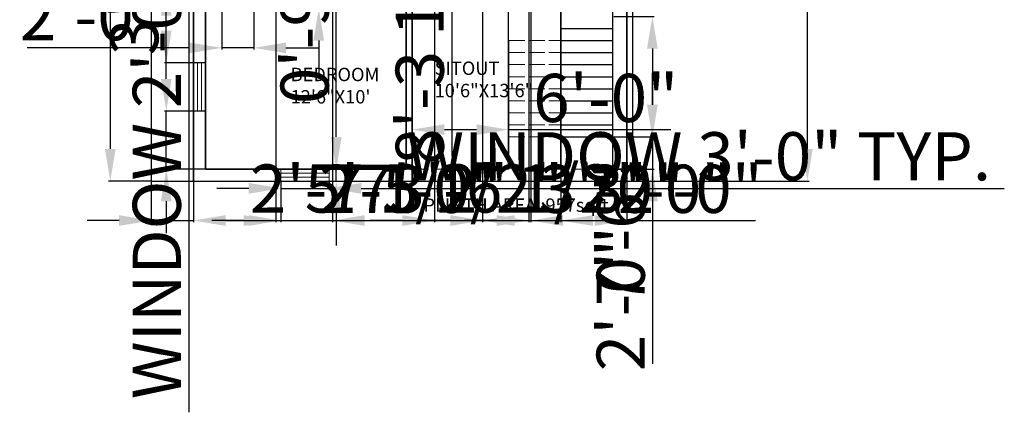
# Model space of a CAD drawing. Units: inches. Extents: x 1041 to 1781, y -140 to 732.
# Tile 1 of 6: x 1045 to 1781, y -140 to 153. Entities that reach past the tile are written whole.
import ezdxf

# ---------------------------------------------------------------- set-up
doc = ezdxf.new("R2010")
doc.units = ezdxf.units.IN
doc.linetypes.add('ACAD_ISO02W100', pattern=[15, 12, -3])
for name, color, linetype, lineweight in [('A-ANNO-TEXT', 7, 'Continuous', 18), ('A-AREA-IDEN', 7, 'Continuous', 20), ('A-FLOR', 7, 'Continuous', 25), ('A-FLOR-HIDN', 7, 'ACAD_ISO02W100', 18), ('A-FLOR-STRS', 7, 'Continuous', 25), ('A-FLOR-STRS-OVHD', 7, 'ACAD_ISO02W100', 18), ('A-GLAZ', 4, 'Continuous', 18), ('A-WALL', 7, 'Continuous', 35), ('C-PROP', 3, 'Continuous', 25), ('dimension', 130, 'Continuous', 18)]:
    doc.layers.add(name, color=color, linetype=linetype, lineweight=lineweight)
doc.styles.get("Standard").update_dxf_attribs({"font": 'arial.ttf'})
doc.dimstyles.new('ISO-25', dxfattribs={"dimtxt": 36, "dimasz": 24, "dimexe": 1.25, "dimexo": 0.625, "dimtad": 1, "dimlunit": 4, "dimtxsty": 'Standard', "dimcen": 2.5, "dimadec": 0, "dimazin": 0, "dimtfac": 1, "dimtmove": 0, "dimatfit": 3, "dimfxl": 1, "dimarcsym": 0})

# ---------------------------------------------------------------- blocks, each defined once
blk = doc.blocks.new('*D2')
at = {"layer": 'Defpoints', "color": 0, "transparency": 16777216}
for p in [(1143.25, 512.23), (1112.63, 32.23), (1143.25, 32.23)]:
    blk.add_point(p, dxfattribs=at)
at = {"layer": 'dimension', "color": 0, "lineweight": -2, "transparency": 16777216}
for p, q in [((1142.62, 512.23), (1111.38, 512.23)), ((1112.63, 488.23), (1112.63, 56.23)), ((1142.62, 32.23), (1111.38, 32.23))]:
    blk.add_line(p, q, dxfattribs=at)
at = {"layer": 'dimension', "color": 0, "transparency": 16777216}
for points in [[(1108.63, 488.23), (1116.63, 488.23), (1112.63, 512.23)], [(1108.63, 56.23), (1116.63, 56.23), (1112.63, 32.23)]]:
    blk.add_solid(points, dxfattribs=at)
at = {"layer": 'dimension', "color": 0, "transparency": 16777216, "insert": (1093.62, 272.23), "char_height": 36, "attachment_point": 5, "rotation": 90}
blk.add_mtext("40'", dxfattribs=at)
blk = doc.blocks.new('WIN-36IN')
for p, q in [((0, 9), (0, 0)), ((36, 9), (0, 9)), ((36, 0), (36, 9)), ((36, 6), (0, 6)), ((0, 3), (36, 3)), ((0, 0), (36, 0)), ((0, 0), (36, 0))]:
    blk.add_line(p, q)
blk = doc.blocks.new('*D9')
at = {"layer": 'Defpoints', "color": 0, "transparency": 16777216}
for p in [(1174.94, 388.32), (1171.34, 364.32), (1174.94, 364.32)]:
    blk.add_point(p, dxfattribs=at)
at = {"layer": 'dimension', "color": 0, "lineweight": -2, "transparency": 16777216}
for p, q in [((1171.34, 412.32), (1171.34, 436.32)), ((1174.31, 388.32), (1170.09, 388.32)), ((1171.34, 388.32), (1171.34, 364.32)), ((1174.31, 364.32), (1170.09, 364.32)), ((1171.34, 340.32), (1171.34, -140.48))]:
    blk.add_line(p, q, dxfattribs=at)
at = {"layer": 'dimension', "color": 0, "transparency": 16777216}
for points in [[(1167.34, 412.32), (1175.34, 412.32), (1171.34, 388.32)], [(1167.34, 340.32), (1175.34, 340.32), (1171.34, 364.32)]]:
    blk.add_solid(points, dxfattribs=at)
at = {"layer": 'dimension', "color": 0, "transparency": 16777216, "insert": (1152.09, 87.92), "char_height": 36, "attachment_point": 5, "rotation": 90}
blk.add_mtext('WINDOW 2\'-0" TYP.', dxfattribs=at)
blk = doc.blocks.new('*D11')
at = {"layer": 'Defpoints', "color": 0, "transparency": 16777216}
for p in [(1240.2, 32.23), (1276.2, 32.23), (1276.2, 26.83)]:
    blk.add_point(p, dxfattribs=at)
at = {"layer": 'dimension', "color": 0, "lineweight": -2, "transparency": 16777216}
for p, q in [((1240.2, 31.61), (1240.2, 25.58)), ((1276.2, 31.61), (1276.2, 25.58)), ((1216.2, 26.83), (1192.2, 26.83)), ((1240.2, 26.83), (1276.2, 26.83)), ((1300.2, 26.83), (1781, 26.83))]:
    blk.add_line(p, q, dxfattribs=at)
at = {"layer": 'dimension', "color": 0, "transparency": 16777216}
for points in [[(1216.2, 30.83), (1216.2, 22.83), (1240.2, 26.83)], [(1300.2, 30.83), (1300.2, 22.83), (1276.2, 26.83)]]:
    blk.add_solid(points, dxfattribs=at)
at = {"layer": 'dimension', "color": 0, "transparency": 16777216, "insert": (1552.6, 46.1), "char_height": 36, "attachment_point": 5}
blk.add_mtext('WINDOW 3\'-0" TYP.', dxfattribs=at)
blk = doc.blocks.new('*D12')
at = {"layer": 'Defpoints', "color": 0, "transparency": 16777216}
for p in [(1276.2, 41.23), (1281.6, 41.23), (1276.2, 32.23)]:
    blk.add_point(p, dxfattribs=at)
at = {"layer": 'dimension', "color": 0, "lineweight": -2, "transparency": 16777216}
for p, q in [((1281.6, 65.23), (1281.6, 309.92)), ((1276.83, 41.23), (1282.85, 41.23)), ((1281.6, 32.23), (1281.6, 41.23)), ((1276.83, 32.23), (1282.85, 32.23)), ((1281.6, 8.23), (1281.6, -15.77))]:
    blk.add_line(p, q, dxfattribs=at)
at = {"layer": 'dimension', "color": 0, "transparency": 16777216}
for points in [[(1277.6, 65.23), (1285.6, 65.23), (1281.6, 41.23)], [(1277.6, 8.23), (1285.6, 8.23), (1281.6, 32.23)]]:
    blk.add_solid(points, dxfattribs=at)
at = {"layer": 'dimension', "color": 0, "transparency": 16777216, "insert": (1262.59, 199.58), "char_height": 36, "attachment_point": 5, "rotation": 90}
blk.add_mtext('0\'-9" TYP.', dxfattribs=at)
blk = doc.blocks.new('*D15')
at = {"layer": 'Defpoints', "color": 0, "transparency": 16777216}
for p in [(1174.94, 32.23), (1498.75, 32.23), (1498.75, 2.78)]:
    blk.add_point(p, dxfattribs=at)
at = {"layer": 'dimension', "color": 0, "lineweight": -2, "transparency": 16777216}
for p, q in [((1174.94, 31.61), (1174.94, 1.53)), ((1498.75, 31.61), (1498.75, 1.53)), ((1198.94, 2.78), (1474.75, 2.78))]:
    blk.add_line(p, q, dxfattribs=at)
at = {"layer": 'dimension', "color": 0, "transparency": 16777216}
for points in [[(1198.94, 6.78), (1198.94, -1.22), (1174.94, 2.78)], [(1474.75, 6.78), (1474.75, -1.22), (1498.75, 2.78)]]:
    blk.add_solid(points, dxfattribs=at)
at = {"layer": 'dimension', "color": 0, "transparency": 16777216, "insert": (1336.84, 21.79), "char_height": 36, "attachment_point": 5}
blk.add_mtext('27\'-0"', dxfattribs=at)
blk = doc.blocks.new('*D16')
at = {"layer": 'Defpoints', "color": 0, "transparency": 16777216}
for p in [(1498.75, 503.23), (1633.79, 503.23), (1498.75, 32.23)]:
    blk.add_point(p, dxfattribs=at)
at = {"layer": 'dimension', "color": 0, "lineweight": -2, "transparency": 16777216}
for p, q in [((1499.37, 503.23), (1635.04, 503.23)), ((1633.79, 56.23), (1633.79, 479.23)), ((1499.37, 32.23), (1635.04, 32.23))]:
    blk.add_line(p, q, dxfattribs=at)
at = {"layer": 'dimension', "color": 0, "transparency": 16777216}
for points in [[(1629.79, 479.23), (1637.79, 479.23), (1633.79, 503.23)], [(1629.79, 56.23), (1637.79, 56.23), (1633.79, 32.23)]]:
    blk.add_solid(points, dxfattribs=at)
at = {"layer": 'dimension', "color": 0, "transparency": 16777216, "insert": (1614.78, 267.73), "char_height": 36, "attachment_point": 5, "rotation": 90}
blk.add_mtext('39\'-3"', dxfattribs=at)
blk = doc.blocks.new('*D17')
at = {"layer": 'Defpoints', "color": 0, "transparency": 16777216}
for p in [(1143.25, 32.23), (1174.94, 32.23), (1174.94, 2.78)]:
    blk.add_point(p, dxfattribs=at)
at = {"layer": 'dimension', "color": 0, "lineweight": -2, "transparency": 16777216}
for p, q in [((1143.25, 31.61), (1143.25, 1.53)), ((1174.94, 31.61), (1174.94, 1.53)), ((1119.25, 2.78), (1095.25, 2.78)), ((1143.25, 2.78), (1174.94, 2.78)), ((1198.94, 2.78), (1404.38, 2.78))]:
    blk.add_line(p, q, dxfattribs=at)
at = {"layer": 'dimension', "color": 0, "transparency": 16777216}
for points in [[(1119.25, 6.78), (1119.25, -1.22), (1143.25, 2.78)], [(1198.94, 6.78), (1198.94, -1.22), (1174.94, 2.78)]]:
    blk.add_solid(points, dxfattribs=at)
at = {"layer": 'dimension', "color": 0, "transparency": 16777216, "insert": (1313.66, 22.02), "char_height": 36, "attachment_point": 5}
blk.add_mtext('2\'-7 1/2"', dxfattribs=at)
blk = doc.blocks.new('*D19')
at = {"layer": 'Defpoints', "color": 0, "transparency": 16777216}
for p in [(1354.94, 447.73), (1390.94, 447.73), (1390.94, 2.78)]:
    blk.add_point(p, dxfattribs=at)
at = {"layer": 'dimension', "color": 0, "lineweight": -2, "transparency": 16777216}
for p, q in [((1354.94, 447.11), (1354.94, 1.53)), ((1390.94, 447.11), (1390.94, 1.53)), ((1330.94, 2.78), (1306.94, 2.78)), ((1354.94, 2.78), (1390.94, 2.78)), ((1414.94, 2.78), (1535.86, 2.78))]:
    blk.add_line(p, q, dxfattribs=at)
at = {"layer": 'dimension', "color": 0, "transparency": 16777216}
for points in [[(1330.94, 6.78), (1330.94, -1.22), (1354.94, 2.78)], [(1414.94, 6.78), (1414.94, -1.22), (1390.94, 2.78)]]:
    blk.add_solid(points, dxfattribs=at)
at = {"layer": 'dimension', "color": 0, "transparency": 16777216, "insert": (1487.4, 21.8), "char_height": 36, "attachment_point": 5}
blk.add_mtext('3\'-0"', dxfattribs=at)
blk = doc.blocks.new('*D20')
at = {"layer": 'Defpoints', "color": 0, "transparency": 16777216}
for p in [(1425.44, 395.23), (1449.44, 395.23), (1449.44, 2.78)]:
    blk.add_point(p, dxfattribs=at)
at = {"layer": 'dimension', "color": 0, "lineweight": -2, "transparency": 16777216}
for p, q in [((1425.44, 394.61), (1425.44, 1.53)), ((1449.44, 394.61), (1449.44, 1.53)), ((1401.44, 2.78), (1377.44, 2.78)), ((1425.44, 2.78), (1449.44, 2.78)), ((1473.44, 2.78), (1595, 2.78))]:
    blk.add_line(p, q, dxfattribs=at)
at = {"layer": 'dimension', "color": 0, "transparency": 16777216}
for points in [[(1401.44, 6.78), (1401.44, -1.22), (1425.44, 2.78)], [(1473.44, 6.78), (1473.44, -1.22), (1449.44, 2.78)]]:
    blk.add_solid(points, dxfattribs=at)
at = {"layer": 'dimension', "color": 0, "transparency": 16777216, "insert": (1546.22, 21.79), "char_height": 36, "attachment_point": 5}
blk.add_mtext('2\'-0"', dxfattribs=at)
blk = doc.blocks.new('*D21')
at = {"layer": 'Defpoints', "color": 0, "transparency": 16777216}
for p in [(1449.44, 541.68), (1410.44, 41.23), (1449.44, 41.23)]:
    blk.add_point(p, dxfattribs=at)
at = {"layer": 'dimension', "color": 0, "lineweight": -2, "transparency": 16777216}
for p, q in [((1386.44, 541.68), (1362.44, 541.68)), ((1410.44, 41.86), (1410.44, 542.93)), ((1410.44, 541.68), (1449.44, 541.68)), ((1449.44, 41.86), (1449.44, 542.93)), ((1473.44, 541.68), (1594.36, 541.68))]:
    blk.add_line(p, q, dxfattribs=at)
at = {"layer": 'dimension', "color": 0, "transparency": 16777216}
for points in [[(1386.44, 545.68), (1386.44, 537.68), (1410.44, 541.68)], [(1473.44, 545.68), (1473.44, 537.68), (1449.44, 541.68)]]:
    blk.add_solid(points, dxfattribs=at)
at = {"layer": 'dimension', "color": 0, "transparency": 16777216, "insert": (1545.9, 560.7), "char_height": 36, "attachment_point": 5}
blk.add_mtext('3\'-3"', dxfattribs=at)
blk = doc.blocks.new('*D22')
at = {"layer": 'Defpoints', "color": 0, "transparency": 16777216}
for p in [(1410.44, 70.68), (1338.44, 41.23), (1410.44, 41.23)]:
    blk.add_point(p, dxfattribs=at)
at = {"layer": 'dimension', "color": 0, "lineweight": -2, "transparency": 16777216}
for p, q in [((1338.44, 41.86), (1338.44, 71.93)), ((1362.44, 70.68), (1386.44, 70.68)), ((1410.44, 41.86), (1410.44, 71.93)), ((1410.44, 70.68), (1531.58, 70.68))]:
    blk.add_line(p, q, dxfattribs=at)
at = {"layer": 'dimension', "color": 0, "transparency": 16777216}
for points in [[(1362.44, 74.68), (1362.44, 66.68), (1338.44, 70.68)], [(1386.44, 74.68), (1386.44, 66.68), (1410.44, 70.68)]]:
    blk.add_solid(points, dxfattribs=at)
at = {"layer": 'dimension', "color": 0, "transparency": 16777216, "insert": (1483.01, 89.69), "char_height": 36, "attachment_point": 5}
blk.add_mtext('6\'-0"', dxfattribs=at)
blk = doc.blocks.new('*D24')
at = {"layer": 'Defpoints', "color": 0, "transparency": 16777216}
for p in [(1154.49, 84.57), (1183.94, 84.57), (1183.94, 41.23)]:
    blk.add_point(p, dxfattribs=at)
at = {"layer": 'dimension', "color": 0, "lineweight": -2, "transparency": 16777216}
for p, q in [((1154.49, 108.57), (1154.49, 313.38)), ((1183.31, 84.57), (1153.24, 84.57)), ((1154.49, 41.23), (1154.49, 84.57)), ((1183.31, 41.23), (1153.24, 41.23)), ((1154.49, 17.23), (1154.49, -6.77))]:
    blk.add_line(p, q, dxfattribs=at)
at = {"layer": 'dimension', "color": 0, "transparency": 16777216}
for points in [[(1150.49, 108.57), (1158.49, 108.57), (1154.49, 84.57)], [(1150.49, 17.23), (1158.49, 17.23), (1154.49, 41.23)]]:
    blk.add_solid(points, dxfattribs=at)
at = {"layer": 'dimension', "color": 0, "transparency": 16777216, "insert": (1135.24, 222.98), "char_height": 36, "attachment_point": 5, "rotation": 90}
blk.add_mtext('3\'-7 1/2"', dxfattribs=at)
blk = doc.blocks.new('*D25')
at = {"layer": 'Defpoints', "color": 0, "transparency": 16777216}
for p in [(1154.49, 179.79), (1183.94, 179.79), (1183.94, 120.57)]:
    blk.add_point(p, dxfattribs=at)
at = {"layer": 'dimension', "color": 0, "lineweight": -2, "transparency": 16777216}
for p, q in [((1154.49, 179.79), (1154.49, 330.15)), ((1183.31, 179.79), (1153.24, 179.79)), ((1154.49, 144.57), (1154.49, 155.79)), ((1183.31, 120.57), (1153.24, 120.57))]:
    blk.add_line(p, q, dxfattribs=at)
at = {"layer": 'dimension', "color": 0, "transparency": 16777216}
for points in [[(1150.49, 155.79), (1158.49, 155.79), (1154.49, 179.79)], [(1150.49, 144.57), (1158.49, 144.57), (1154.49, 120.57)]]:
    blk.add_solid(points, dxfattribs=at)
at = {"layer": 'dimension', "color": 0, "transparency": 16777216, "insert": (1135.79, 266.97), "char_height": 36, "attachment_point": 5, "rotation": 90}
blk.add_mtext('4\'-11"', dxfattribs=at)
blk = doc.blocks.new('*D30')
at = {"layer": 'Defpoints', "color": 0, "transparency": 16777216}
for p in [(1174.94, 32.23), (1240.2, 32.23), (1240.2, 2.78)]:
    blk.add_point(p, dxfattribs=at)
at = {"layer": 'dimension', "color": 0, "lineweight": -2, "transparency": 16777216}
for p, q in [((1174.94, 31.61), (1174.94, 1.53)), ((1240.2, 31.61), (1240.2, 1.53)), ((1198.94, 2.78), (1216.2, 2.78)), ((1240.2, 2.78), (1445.03, 2.78))]:
    blk.add_line(p, q, dxfattribs=at)
at = {"layer": 'dimension', "color": 0, "transparency": 16777216}
for points in [[(1198.94, 6.78), (1198.94, -1.22), (1174.94, 2.78)], [(1216.2, 6.78), (1216.2, -1.22), (1240.2, 2.78)]]:
    blk.add_solid(points, dxfattribs=at)
at = {"layer": 'dimension', "color": 0, "transparency": 16777216, "insert": (1354.62, 22.02), "char_height": 36, "attachment_point": 5}
blk.add_mtext('5\'-5 1/2"', dxfattribs=at)
blk = doc.blocks.new('*D31')
at = {"layer": 'Defpoints', "color": 0, "transparency": 16777216}
for p in [(1390.94, 447.73), (1427, 447.73), (1427, 2.78)]:
    blk.add_point(p, dxfattribs=at)
at = {"layer": 'dimension', "color": 0, "lineweight": -2, "transparency": 16777216}
for p, q in [((1390.94, 447.11), (1390.94, 1.53)), ((1427, 447.11), (1427, 1.53)), ((1366.94, 2.78), (1342.94, 2.78)), ((1390.94, 2.78), (1427, 2.78)), ((1451, 2.78), (1571.93, 2.78))]:
    blk.add_line(p, q, dxfattribs=at)
at = {"layer": 'dimension', "color": 0, "transparency": 16777216}
for points in [[(1366.94, 6.78), (1366.94, -1.22), (1390.94, 2.78)], [(1451, 6.78), (1451, -1.22), (1427, 2.78)]]:
    blk.add_solid(points, dxfattribs=at)
at = {"layer": 'dimension', "color": 0, "transparency": 16777216, "insert": (1523.46, 21.8), "char_height": 36, "attachment_point": 5}
blk.add_mtext('3\'-0"', dxfattribs=at)
blk = doc.blocks.new('*D32')
at = {"layer": 'Defpoints', "color": 0, "transparency": 16777216}
for p in [(1236.44, 447.73), (1278.74, 447.73), (1278.74, 2.78)]:
    blk.add_point(p, dxfattribs=at)
at = {"layer": 'dimension', "color": 0, "lineweight": -2, "transparency": 16777216}
for p, q in [((1236.44, 447.11), (1236.44, 1.53)), ((1278.74, 447.11), (1278.74, 1.53)), ((1212.44, 2.78), (1188.44, 2.78)), ((1236.44, 2.78), (1278.74, 2.78)), ((1302.74, 2.78), (1507.55, 2.78))]:
    blk.add_line(p, q, dxfattribs=at)
at = {"layer": 'dimension', "color": 0, "transparency": 16777216}
for points in [[(1212.44, 6.78), (1212.44, -1.22), (1236.44, 2.78)], [(1302.74, 6.78), (1302.74, -1.22), (1278.74, 2.78)]]:
    blk.add_solid(points, dxfattribs=at)
at = {"layer": 'dimension', "color": 0, "transparency": 16777216, "insert": (1417.15, 22.03), "char_height": 36, "attachment_point": 5}
blk.add_mtext('3\'-6 1/2"', dxfattribs=at)
blk = doc.blocks.new('*D33')
at = {"layer": 'Defpoints', "color": 0, "transparency": 16777216}
for p in [(1488.44, 155.23), (1488.44, 65.23), (1517.89, 65.23)]:
    blk.add_point(p, dxfattribs=at)
at = {"layer": 'dimension', "color": 0, "lineweight": -2, "transparency": 16777216}
for p, q in [((1489.06, 155.23), (1519.14, 155.23)), ((1517.89, 131.23), (1517.89, 89.23)), ((1489.06, 65.23), (1519.14, 65.23)), ((1517.89, 65.23), (1517.89, -55.42))]:
    blk.add_line(p, q, dxfattribs=at)
at = {"layer": 'dimension', "color": 0, "transparency": 16777216}
for points in [[(1513.89, 131.23), (1521.89, 131.23), (1517.89, 155.23)], [(1513.89, 89.23), (1521.89, 89.23), (1517.89, 65.23)]]:
    blk.add_solid(points, dxfattribs=at)
at = {"layer": 'dimension', "color": 0, "transparency": 16777216, "insert": (1498.88, -7.09), "char_height": 36, "attachment_point": 5, "rotation": 90}
blk.add_mtext('7\'-6"', dxfattribs=at)
blk = doc.blocks.new('*D36')
at = {"layer": 'Defpoints', "color": 0, "transparency": 16777216}
for p in [(1195.94, 161.23), (1219.94, 161.23), (1195.94, 131.78)]:
    blk.add_point(p, dxfattribs=at)
at = {"layer": 'dimension', "color": 0, "lineweight": -2, "transparency": 16777216}
for p, q in [((1195.94, 160.61), (1195.94, 130.53)), ((1219.94, 160.61), (1219.94, 130.53)), ((1171.94, 131.78), (1050.38, 131.78)), ((1219.94, 131.78), (1195.94, 131.78)), ((1243.94, 131.78), (1267.94, 131.78))]:
    blk.add_line(p, q, dxfattribs=at)
at = {"layer": 'dimension', "color": 0, "transparency": 16777216}
for points in [[(1171.94, 135.78), (1171.94, 127.78), (1195.94, 131.78)], [(1243.94, 135.78), (1243.94, 127.78), (1219.94, 131.78)]]:
    blk.add_solid(points, dxfattribs=at)
at = {"layer": 'dimension', "color": 0, "transparency": 16777216, "insert": (1099.16, 150.79), "char_height": 36, "attachment_point": 5}
blk.add_mtext('2\'-0"', dxfattribs=at)
blk = doc.blocks.new('*D41')
at = {"layer": 'Defpoints', "color": 0, "transparency": 16777216}
for p in [(1268.49, 165.73), (1297.94, 165.73), (1297.94, 161.23)]:
    blk.add_point(p, dxfattribs=at)
at = {"layer": 'dimension', "color": 0, "lineweight": -2, "transparency": 16777216}
for p, q in [((1268.49, 189.73), (1268.49, 394.57)), ((1297.31, 165.73), (1267.24, 165.73)), ((1268.49, 161.23), (1268.49, 165.73)), ((1297.31, 161.23), (1267.24, 161.23)), ((1268.49, 137.23), (1268.49, 113.23))]:
    blk.add_line(p, q, dxfattribs=at)
at = {"layer": 'dimension', "color": 0, "transparency": 16777216}
for points in [[(1264.49, 189.73), (1272.49, 189.73), (1268.49, 165.73)], [(1264.49, 137.23), (1272.49, 137.23), (1268.49, 161.23)]]:
    blk.add_solid(points, dxfattribs=at)
at = {"layer": 'dimension', "color": 0, "transparency": 16777216, "insert": (1249.25, 304.15), "char_height": 36, "attachment_point": 5, "rotation": 90}
blk.add_mtext('0\'-4 1/2"', dxfattribs=at)
blk = doc.blocks.new('*D42')
at = {"layer": 'Defpoints', "color": 0, "transparency": 16777216}
for p in [(1488.44, 65.23), (1488.44, 41.23), (1517.89, 41.23)]:
    blk.add_point(p, dxfattribs=at)
at = {"layer": 'dimension', "color": 0, "lineweight": -2, "transparency": 16777216}
for p, q in [((1517.89, 89.23), (1517.89, 113.23)), ((1489.06, 65.23), (1519.14, 65.23)), ((1517.89, 65.23), (1517.89, 41.23)), ((1489.06, 41.23), (1519.14, 41.23)), ((1517.89, 17.23), (1517.89, -104.33))]:
    blk.add_line(p, q, dxfattribs=at)
at = {"layer": 'dimension', "color": 0, "transparency": 16777216}
for points in [[(1513.89, 89.23), (1521.89, 89.23), (1517.89, 65.23)], [(1513.89, 17.23), (1521.89, 17.23), (1517.89, 41.23)]]:
    blk.add_solid(points, dxfattribs=at)
at = {"layer": 'dimension', "color": 0, "transparency": 16777216, "insert": (1498.88, -55.55), "char_height": 36, "attachment_point": 5, "rotation": 90}
blk.add_mtext('2\'-0"', dxfattribs=at)
blk = doc.blocks.new('*D44')
at = {"layer": 'Defpoints', "color": 0, "transparency": 16777216}
for p in [(1338.44, 354.73), (1338.44, 255.41), (1367.89, 255.41)]:
    blk.add_point(p, dxfattribs=at)
at = {"layer": 'dimension', "color": 0, "lineweight": -2, "transparency": 16777216}
for p, q in [((1339.06, 354.73), (1369.14, 354.73)), ((1367.89, 330.73), (1367.89, 279.41)), ((1339.06, 255.41), (1369.14, 255.41)), ((1367.89, 255.41), (1367.89, 50.53))]:
    blk.add_line(p, q, dxfattribs=at)
at = {"layer": 'dimension', "color": 0, "transparency": 16777216}
for points in [[(1363.89, 330.73), (1371.89, 330.73), (1367.89, 354.73)], [(1363.89, 279.41), (1371.89, 279.41), (1367.89, 255.41)]]:
    blk.add_solid(points, dxfattribs=at)
at = {"layer": 'dimension', "color": 0, "transparency": 16777216, "insert": (1348.64, 140.97), "char_height": 36, "attachment_point": 5, "rotation": 90}
blk.add_mtext('8\'-3 1/2"', dxfattribs=at)

msp = doc.modelspace()

# ---------------------------------------------------------------- linework, layer by layer
at = {"layer": 'A-FLOR'}
msp.add_line((1488.438, 32.233), (1488.438, 203.233), dxfattribs=at)
at = {"layer": 'A-FLOR-HIDN'}
msp.add_line((1338.438, 41.233), (1488.438, 41.233), dxfattribs=at)
at = {"layer": 'A-FLOR-STRS'}
for p, q in [((1449.438, 155.233), (1449.438, 41.233)), ((1449.438, 146.233), (1488.438, 146.233)), ((1410.438, 137.233), (1410.438, 41.233)), ((1449.438, 137.233), (1488.438, 137.233)), ((1449.438, 128.233), (1488.438, 128.233)), ((1449.438, 119.233), (1488.438, 119.233)), ((1449.438, 110.233), (1488.438, 110.233)), ((1449.438, 101.233), (1488.438, 101.233)), ((1449.438, 92.233), (1488.438, 92.233)), ((1449.438, 83.233), (1488.438, 83.233)), ((1449.438, 74.233), (1488.438, 74.233)), ((1449.438, 65.233), (1488.438, 65.233))]:
    msp.add_line(p, q, dxfattribs=at)
at = {"layer": 'A-FLOR-STRS-OVHD'}
for p, q in [((1410.438, 137.233), (1449.438, 137.233)), ((1410.438, 128.233), (1449.438, 128.233)), ((1410.438, 119.233), (1449.438, 119.233)), ((1410.438, 110.233), (1449.438, 110.233)), ((1410.438, 101.233), (1449.438, 101.233)), ((1410.438, 92.233), (1449.438, 92.233)), ((1410.438, 83.233), (1449.438, 83.233)), ((1410.438, 74.233), (1449.438, 74.233)), ((1410.438, 65.233), (1449.438, 65.233))]:
    msp.add_line(p, q, dxfattribs=at)
at = {"layer": 'A-WALL'}
for p, q in [((1498.749, 32.233), (1498.749, 512.233)), ((1174.938, 41.233), (1174.938, 503.233)), ((1338.438, 41.233), (1338.438, 203.233)), ((1183.938, 41.233), (1183.938, 161.233)), ((1333.938, 41.233), (1333.938, 161.233)), ((1174.938, 41.233), (1174.938, 32.233)), ((1183.938, 41.233), (1333.938, 41.233)), ((1338.438, 41.233), (1338.438, 32.233)), ((1488.438, 41.233), (1498.749, 41.233))]:
    msp.add_line(p, q, dxfattribs=at)
at = {"layer": 'C-PROP'}
for p, q in [((1143.249, 512.233), (1143.249, 32.233)), ((1503.249, 32.233), (1503.249, 512.233)), ((1143.249, 32.233), (1503.249, 32.233))]:
    msp.add_line(p, q, dxfattribs=at)

# ---------------------------------------------------------------- block references
at = {"layer": 'A-GLAZ', "rotation": 89.9999999999994}
msp.add_blockref('WIN-36IN', (1183.937, 84.573), dxfattribs=at)
at = {"layer": 'A-GLAZ'}
msp.add_blockref('WIN-36IN', (1240.201, 32.233), dxfattribs=at)

# ---------------------------------------------------------------- texts
at = {"layer": 'A-ANNO-TEXT', "insert": (1346.752, 19.286), "char_height": 10, "attachment_point": 1}
msp.add_mtext_dynamic_manual_height_columns('PLINTH AREA :957sqft', width=169.36465, gutter_width=12.5, heights=[0], dxfattribs=at)
at = {"layer": 'A-AREA-IDEN', "char_height": 10, "attachment_point": 1}
for s, insert in [('SITOUT\\P10\'6"X13\'6"', (1355.113, 121.561)), ('BEDROOM\\P12\'6"X10\'', (1247.439, 116.884))]:
    msp.add_mtext_dynamic_manual_height_columns(s, width=64.5482, gutter_width=12.5, heights=[0], dxfattribs=dict(at, insert=insert))

# ---------------------------------------------------------------- dimensions: what is measured, and where the dimension line sits
at = {"layer": 'dimension'}
for base, p1, p2, picture, middle in [((1449.438, 541.683), (1410.438, 41.233), (1449.438, 41.233), '*D21', (1545.899, 560.7)), ((1278.743, 2.783), (1236.438, 447.733), (1278.743, 447.733), '*D32', (1417.147, 22.034)), ((1390.938, 2.783), (1354.938, 447.733), (1390.938, 447.733), '*D19', (1487.399, 21.8)), ((1427.003, 2.783), (1390.938, 447.733), (1427.003, 447.733), '*D31', (1523.464, 21.8)), ((1449.438, 2.783), (1425.438, 395.233), (1449.438, 395.233), '*D20', (1546.218, 21.788)), ((1410.438, 70.683), (1338.438, 41.233), (1410.438, 41.233), '*D22', (1483.009, 89.688)), ((1174.938, 2.783), (1143.249, 32.233), (1174.938, 32.233), '*D17', (1313.661, 22.021)), ((1240.201, 2.783), (1174.938, 32.233), (1240.201, 32.233), '*D30', (1354.617, 22.021)), ((1498.749, 2.783), (1174.938, 32.233), (1498.749, 32.233), '*D15', (1336.843, 21.788))]:
    dim = msp.add_linear_dim(base=base, p1=p1, p2=p2, dimstyle='ISO-25', override={"dimdec": 1, "dimlfac": 1, "dimrnd": 0, "dimzin": 1, "dimdsep": 46, "dimlunit": 4, "dimfrac": 2}, dxfattribs=at)
    dim.commit()
    dim.dimension.update_dxf_attribs({"geometry": picture, "text_midpoint": middle})
for base, p1, p2, angle, override, picture, middle in [((1112.63, 32.233), (1143.249, 512.233), (1143.249, 32.233), 90, {"dimclrd": 0, "dimclre": 0, "dimclrt": 0}, '*D2', (1093.625, 272.233)), ((1633.794, 503.233), (1498.749, 32.233), (1498.749, 503.233), 90, {"dimdec": 1, "dimlfac": 1, "dimrnd": 0, "dimzin": 1, "dimdsep": 46, "dimlunit": 4, "dimfrac": 2}, '*D16', (1614.777, 267.733)), ((1268.488, 165.733), (1297.938, 161.233), (1297.938, 165.733), 90, {"dimdec": 1, "dimlfac": 1, "dimrnd": 0, "dimzin": 1, "dimdsep": 46, "dimlunit": 4, "dimfrac": 2}, '*D41', (1249.249, 304.149)), ((1367.888, 255.408), (1338.438, 354.733), (1338.438, 255.408), 270, {"dimdec": 1, "dimlfac": 1, "dimrnd": 0, "dimzin": 1, "dimdsep": 46, "dimlunit": 4, "dimfrac": 2}, '*D44', (1348.636, 140.967)), ((1154.488, 179.788), (1183.938, 120.573), (1183.938, 179.788), 90, {"dimdec": 1, "dimlfac": 1, "dimrnd": 0, "dimzin": 1, "dimdsep": 46, "dimlunit": 4, "dimfrac": 2}, '*D25', (1135.789, 266.971)), ((1154.488, 84.573), (1183.938, 41.233), (1183.938, 84.573), 90, {"dimdec": 1, "dimlfac": 1, "dimrnd": 0, "dimzin": 1, "dimdsep": 46, "dimlunit": 4, "dimfrac": 2}, '*D24', (1135.236, 222.977)), ((1195.938, 131.783), (1219.938, 161.233), (1195.938, 161.233), 180, {"dimdec": 1, "dimlfac": 1, "dimrnd": 0, "dimzin": 1, "dimdsep": 46, "dimlunit": 4, "dimfrac": 2}, '*D36', (1099.157, 150.788)), ((1517.888, 65.233), (1488.438, 155.233), (1488.438, 65.233), 270, {"dimdec": 1, "dimlfac": 1, "dimrnd": 0, "dimzin": 1, "dimdsep": 46, "dimlunit": 4, "dimfrac": 2}, '*D33', (1498.882, -7.094)), ((1517.888, 41.233), (1488.438, 65.233), (1488.438, 41.233), 270, {"dimdec": 1, "dimlfac": 1, "dimrnd": 0, "dimzin": 1, "dimdsep": 46, "dimlunit": 4, "dimfrac": 2}, '*D42', (1498.882, -55.548))]:
    dim = msp.add_linear_dim(base=base, p1=p1, p2=p2, angle=angle, dimstyle='ISO-25', override=override, dxfattribs=at)
    dim.commit()
    dim.dimension.update_dxf_attribs({"geometry": picture, "text_midpoint": middle})
for base, p1, p2, angle, text, picture, middle in [((1171.338, 364.318), (1174.938, 388.318), (1174.938, 364.318), 270, 'WINDOW <> TYP.', '*D9', (1152.086, 87.918)), ((1281.601, 41.233), (1276.201, 32.233), (1276.201, 41.233), 90, '<> TYP.', '*D12', (1262.595, 199.577))]:
    dim = msp.add_linear_dim(base=base, p1=p1, p2=p2, angle=angle, text=text, dimstyle='ISO-25', override={"dimdec": 1, "dimlfac": 1, "dimrnd": 0, "dimzin": 1, "dimdsep": 46, "dimlunit": 4, "dimfrac": 2}, dxfattribs=at)
    dim.commit()
    dim.dimension.update_dxf_attribs({"geometry": picture, "text_midpoint": middle})
dim = msp.add_linear_dim(base=(1276.201, 26.833), p1=(1240.201, 32.233), p2=(1276.201, 32.233), text='WINDOW <> TYP.', dimstyle='ISO-25', override={"dimdec": 1, "dimlfac": 1, "dimrnd": 0, "dimzin": 1, "dimdsep": 46, "dimlunit": 4, "dimfrac": 2}, dxfattribs=at)
dim.commit()
dim.dimension.update_dxf_attribs({"geometry": '*D11', "text_midpoint": (1552.6, 46.096)})

doc.saveas('drawing.dxf')
